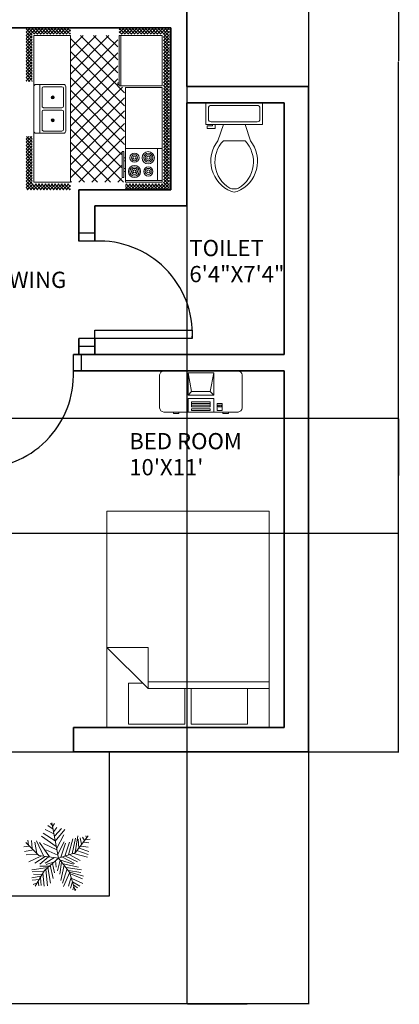
# Model space of a CAD drawing. Units: inches. Extents: x 4159 to 4826, y 299 to 1026.
# Tile 34 of 37: x 4685 to 4826, y 299 to 663. Entities that reach past the tile are written whole.
import ezdxf

# ---------------------------------------------------------------- set-up
doc = ezdxf.new("R2010")
doc.units = ezdxf.units.IN
for name, color, linetype, lineweight in [('A-ANNO-DIMS', 2, 'Continuous', 18), ('A-AREA-IDEN', 7, 'Continuous', 18), ('A-DOOR', 4, 'Continuous', 25), ('A-EQPM', 8, 'Continuous', 13), ('A-FLOR-BALC', 7, 'Continuous', 25), ('A-FLOR-FIXT', 9, 'Continuous', 18), ('A-FURN', 8, 'Continuous', 18), ('A-WALL', 7, 'Continuous', 35), ('L-PLNT', 94, 'Continuous', 13)]:
    doc.layers.add(name, color=color, linetype=linetype, lineweight=lineweight)
doc.styles.get("Standard").update_dxf_attribs({"font": 'arial.ttf'})
doc.dimstyles.get("Standard").update_dxf_attribs({"dimtxt": 0.18, "dimasz": 0.18, "dimexe": 0.18, "dimexo": 0.0625, "dimgap": 0.09, "dimtad": 0, "dimtih": 1, "dimtoh": 1, "dimdec": 4, "dimzin": 0, "dimdsep": 46, "dimtxsty": 'Standard', "dimcen": 0.09, "dimadec": 0, "dimazin": 0, "dimtfac": 1, "dimtdec": 4, "dimtofl": 0, "dimtmove": 0, "dimatfit": 3, "dimfxl": 1, "dimtolj": 1, "dimtzin": 0, "dimarcsym": 0})

# ---------------------------------------------------------------- blocks, each defined once
blk = doc.blocks.new('Bed - Queen')
for p, q in [((0, -80.00003), (0, 0)), ((0, 0), (59.99999, 0)), ((59.99999, 0), (59.99999, -80.00003)), ((7.99999, -1.2), (28.79998, -1.2)), ((7.99999, -14.4), (7.99999, -1.2)), ((28.79998, -1.2), (28.79998, -14.4)), ((31.19999, -1.2), (51.99999, -1.2)), ((31.19999, -14.4), (31.19999, -1.2)), ((51.99999, -1.2), (51.99999, -16.4)), ((0, -14.4), (44.8, -14.4)), ((59.99999, -29.6), (44.8, -14.4)), ((44.8, -14.4), (44.8, -29.6)), ((44.8, -16.8), (0, -16.8)), ((51.99999, -16.4), (46.79936, -16.4)), ((44.8, -29.6), (59.99999, -29.6)), ((59.99999, -80.00003), (0, -80.00003))]:
    blk.add_line(p, q)
blk = doc.blocks.new('Toilet - top')
for p, q in [((9.5, -6), (9.5, -2)), ((-10, -8.5), (-8, -8.5)), ((-10, -9.5), (-10, -8.5)), ((-7, -9.5), (-10, -9.5)), ((-8, -8.5), (-8, -8)), ((-7, -8), (-7, -9.5)), ((-4, -8), (-6, -14)), ((4, -8), (6, -14)), ((4, -14), (-4, -14))]:
    blk.add_line(p, q)
blk.add_lwpolyline([(10.5, -8), (10.5, 0), (-10.5, 0), (-10.5, -8)], close=True)
for points in [[(-9.5, -2), (-9.5, -6)], [(8.5, -1), (-8.5, -1)], [(-8.5, -7), (8.5, -7)]]:
    blk.add_lwpolyline(points)
for centre, radius, start, end in [((-8.62, -1.88), 0.884, 81.8699, 188.1301), ((8.62, -1.88), 0.884, 351.8699, 98.1301), ((-8.62, -6.12), 0.884, 171.8699, 278.1301), ((8.62, -6.12), 0.884, 261.8699, 8.1301), ((3.52, -21.58), 12.17, 141.4691, 247.9714), ((4.2, -21.82), 11.33, 136.3677, 238.9468), ((-3.52, -21.58), 12.17, 292.0284, 38.5307), ((-4.2, -21.82), 11.33, 301.053, 43.6321), ((0, -27.88), 4, 245.7318, 294.2682), ((0, -29), 4, 254.8605, 285.1395)]:
    blk.add_arc(centre, radius, start, end)
blk = doc.blocks.new('Desk - 30 x 60 in.')
for p, q in [((-26.999995, 0), (26.999995, 0)), ((-29.999995, -27), (-29.999995, -3)), ((29.999995, -3), (29.999995, -27)), ((26.999995, -30), (-26.999995, -30)), ((-20.000005, -30), (-20.000005, -31)), ((-20.000005, -31), (-16.000005, -31)), ((-16.000005, -31), (-16.000005, -30)), ((15.999995, -31), (15.999995, -30)), ((19.999995, -31), (15.999995, -31)), ((19.999995, -30), (19.999995, -31))]:
    blk.add_line(p, q)
for centre, start, end in [((-26.499995, -3.5), 98.1301, 171.8699), ((26.499995, -3.5), 8.130102, 81.8699), ((-26.499995, -26.5), 188.1301, 261.8699), ((26.499995, -26.5), 278.1301, 351.8699)]:
    blk.add_arc(centre, 3.535534, start, end)
blk = doc.blocks.new('Computer Terminal')
for p, q in [((-10, 11.5), (5, 11.5)), ((-8, 0.5), (-10, 11.5)), ((-10, -1.5), (-10, 11.5)), ((5, 11.5), (3, 0.5)), ((5, 11.5), (5, -1.5)), ((-10, -1.5), (-8, 0.5)), ((3, 0.5), (-8, 0.5)), ((3, 0.5), (5, -1.5)), ((5, -1.5), (-10, -1.5)), ((-10, -11.5), (-10, -3.5)), ((-10, -3.5), (5, -3.5)), ((-8, -5.5), (-8, -8.5)), ((3, -5.5), (-8, -5.5)), ((3, -8.5), (3, -5.5)), ((5, -3.5), (5, -11.5)), ((5, -11.5), (-10, -11.5)), ((3, -6.5), (-8, -6.5)), ((-8, -7.5), (3, -7.5)), ((-8, -8.5), (3, -8.5)), ((-8, -9.5), (-8, -10.5)), ((3, -9.5), (-8, -9.5)), ((-8, -10.5), (3, -10.5)), ((3, -10.5), (3, -9.5)), ((10, -6.5), (7, -6.5)), ((7, -6.5), (7, -10.5)), ((7, -10.5), (10, -10.5)), ((9.5, -7.5), (7.5, -7.5)), ((7.5, -7.5), (7.5, -8.5)), ((7.5, -8.5), (9.5, -8.5)), ((8.5, -7.5), (8.5, -8.5)), ((9.5, -8.5), (9.5, -7.5)), ((10, -10.5), (10, -6.5))]:
    blk.add_line(p, q)
blk = doc.blocks.new('Kitchen Layout - 7 x 8 ft')
for p, q in [((-5, 81.32), (2.68, 89)), ((-5, 83.44), (0.56, 89)), ((-5, 85.56), (-1.56, 89)), ((-5, 87.68), (-3.68, 89)), ((-1, 84.97), (-5, 88.97)), ((-1, 82.85), (-5, 86.85)), ((-1, 80.73), (-5, 84.73)), ((1.09, 85), (-2.91, 89)), ((3.21, 85), (-0.79, 89)), ((0.81, 85), (4.81, 89)), ((5.34, 85), (1.34, 89)), ((2.93, 85), (6.93, 89)), ((7.46, 85), (3.46, 89)), ((5.05, 85), (9.05, 89)), ((9.58, 85), (5.58, 89)), ((7.17, 85), (11.17, 89)), ((11.7, 85), (7.7, 89)), ((9.29, 85), (13.29, 89)), ((13.82, 85), (9.82, 89)), ((11.41, 85), (15.41, 89)), ((15.94, 85), (11.94, 89)), ((13.53, 85), (17.53, 89)), ((18.06, 85), (14.06, 89)), ((15.65, 85), (19.65, 89)), ((20.18, 85), (16.18, 89)), ((17.78, 85), (21.78, 89)), ((22.31, 85), (18.31, 89)), ((19.9, 85), (23.9, 89)), ((24.43, 85), (20.43, 89)), ((22.02, 85), (26.02, 89)), ((26.55, 85), (22.55, 89)), ((24.14, 85), (28.14, 89)), ((28.67, 85), (24.67, 89)), ((26.26, 85), (30.26, 89)), ((30.79, 85), (26.79, 89)), ((28.38, 85), (32.38, 89)), ((32.91, 85), (28.91, 89)), ((30.5, 85), (34.5, 89)), ((35.03, 85), (31.03, 89)), ((32.63, 85), (36.63, 89)), ((37.16, 85), (33.16, 89)), ((34, 84), (96, 84)), ((34, 60), (34, 84)), ((34.75, 85), (38.75, 89)), ((39.28, 85), (35.28, 89)), ((36.87, 85), (40.87, 89)), ((41.4, 85), (37.4, 89)), ((38.99, 85), (42.99, 89)), ((43.52, 85), (39.52, 89)), ((41.11, 85), (45.11, 89)), ((45.64, 85), (41.64, 89)), ((43.23, 85), (47.23, 89)), ((47.76, 85), (43.76, 89)), ((45.35, 85), (49.35, 89)), ((49.88, 85), (45.88, 89)), ((47.47, 85), (51.47, 89)), ((52, 85), (48, 89)), ((49.6, 85), (53.6, 89)), ((54.13, 85), (50.13, 89)), ((51.72, 85), (55.72, 89)), ((56.25, 85), (52.25, 89)), ((53.84, 85), (57.84, 89)), ((58.37, 85), (54.37, 89)), ((55.96, 85), (59.96, 89)), ((60.49, 85), (56.49, 89)), ((58.08, 85), (62.08, 89)), ((62.61, 85), (58.61, 89)), ((60.2, 85), (64.2, 89)), ((64.73, 85), (60.73, 89)), ((62.32, 85), (66.32, 89)), ((66.85, 85), (62.85, 89)), ((64.45, 85), (68.45, 89)), ((68.97, 85), (64.97, 89)), ((66.57, 85), (70.57, 89)), ((71.1, 85), (67.1, 89)), ((68.69, 85), (72.69, 89)), ((73.22, 85), (69.22, 89)), ((70.81, 85), (74.81, 89)), ((75.34, 85), (71.34, 89)), ((72.93, 85), (76.93, 89)), ((77.46, 85), (73.46, 89)), ((75.05, 85), (79.05, 89)), ((79.58, 85), (75.58, 89)), ((77.17, 85), (81.17, 89)), ((81.7, 85), (77.7, 89)), ((79.29, 85), (83.29, 89)), ((83.82, 85), (79.82, 89)), ((81.42, 85), (85.42, 89)), ((85.95, 85), (81.95, 89)), ((83.54, 85), (87.54, 89)), ((88.07, 85), (84.07, 89)), ((85.66, 85), (89.66, 89)), ((90.19, 85), (86.19, 89)), ((87.78, 85), (91.78, 89)), ((92.31, 85), (88.31, 89)), ((89.9, 85), (93.9, 89)), ((94.43, 85), (90.43, 89)), ((92.02, 85), (96.02, 89)), ((96.55, 85), (92.55, 89)), ((94.14, 85), (98.14, 89)), ((101, 82.67), (94.67, 89)), ((96, 84), (96, 60)), ((96.27, 85), (100.27, 89)), ((101, 84.79), (96.79, 89)), ((97, 83.61), (101, 87.61)), ((97, 81.49), (101, 85.49)), ((101, 80.55), (97, 84.55)), ((101, 86.92), (98.92, 89)), ((-5, 79.19), (-1, 83.19)), ((-1, 78.61), (-5, 82.61)), ((-5, 77.07), (-1, 81.07)), ((-1, 76.49), (-5, 80.49)), ((-5, 74.95), (-1, 78.95)), ((-1, 74.36), (-5, 78.36)), ((74, 81), (95, 81)), ((97, 79.37), (101, 83.37)), ((101, 78.43), (97, 82.43)), ((97, 77.25), (101, 81.25)), ((101, 76.31), (97, 80.31)), ((97, 75.13), (101, 79.13)), ((101, 74.19), (97, 78.19)), ((-5, 72.83), (-1, 76.83)), ((-1, 72.24), (-5, 76.24)), ((-5, 70.71), (-1, 74.71)), ((-1, 70.12), (-5, 74.12)), ((-5, 68.59), (-1, 72.59)), ((-1, 68), (-5, 72)), ((97, 73.01), (101, 77.01)), ((101, 72.07), (97, 76.07)), ((97, 70.89), (101, 74.89)), ((101, 69.95), (97, 73.95)), ((97, 68.76), (101, 72.76)), ((101, 67.82), (97, 71.82)), ((-5, 66.47), (-1, 70.47)), ((-1, 65.88), (-5, 69.88)), ((-5, 64.35), (-1, 68.35)), ((-1, 63.76), (-5, 67.76)), ((-5, 62.22), (-1, 66.22)), ((-1, 61.64), (-5, 65.64)), ((97, 66.64), (101, 70.64)), ((101, 65.7), (97, 69.7)), ((97, 64.52), (101, 68.52)), ((101, 63.58), (97, 67.58)), ((97, 62.4), (101, 66.4)), ((101, 61.46), (97, 65.46)), ((-5, 60.1), (-1, 64.1)), ((-1, 59.52), (-5, 63.52)), ((-5, 57.98), (-1, 61.98)), ((-1, 57.39), (-5, 61.39)), ((-1.73, 56), (-5, 59.27)), ((-4.86, 56), (-1, 59.86)), ((10.4, 24), (45.9, 59.5)), ((18.88, 24), (54.38, 59.5)), ((27.37, 24), (62.87, 59.5)), ((33.03, 55.11), (37.41, 59.5)), ((96, 60), (34, 60)), ((35.85, 24), (71.35, 59.5)), ((76.2, 24), (40.7, 59.5)), ((84.68, 24), (49.18, 59.5)), ((93.17, 24), (57.67, 59.5)), ((61.31, 24), (96, 58.69)), ((96, 29.65), (66.15, 59.5)), ((80, 60), (80, 59)), ((82, 59), (82, 60)), ((87, 59), (87, 60)), ((89, 60), (89, 59)), ((97, 60.28), (101, 64.28)), ((100.34, 60), (97, 63.34)), ((98.22, 60), (97, 61.22)), ((98.84, 60), (101, 62.16)), ((100.96, 60), (101, 60.04)), ((-3.85, 56), (-5, 57.15)), ((-2.74, 56), (-1, 57.74)), ((0, 57), (33, 57)), ((0, 30.57), (24.43, 55)), ((0, 39.06), (15.94, 55)), ((0, 47.54), (7.46, 55)), ((1.91, 24), (32.91, 55)), ((33.77, 24), (2.77, 55)), ((42.26, 24), (11.26, 55)), ((50.74, 24), (19.74, 55)), ((59.23, 24), (28.23, 55)), ((31, 55), (31, 56)), ((32, 55), (31, 55)), ((32, 56), (32, 55)), ((67.71, 24), (33.68, 58.04)), ((44.34, 24), (77.84, 57.5)), ((52.82, 24), (86.32, 57.5)), ((96, 38.14), (76.64, 57.5)), ((96, 46.63), (85.13, 57.5)), ((96, 55.11), (93.57, 57.54)), ((25.29, 24), (0, 49.29)), ((69.79, 24), (96, 50.21)), ((16.8, 24), (0, 40.8)), ((78.28, 24), (96, 41.72)), ((8.32, 24), (0, 32.32)), ((86.76, 24), (96, 33.24)), ((-5, 21.92), (-2.92, 24)), ((-5, 19.8), (-1, 23.8)), ((-1, 19.21), (-5, 23.21)), ((-5, 17.68), (-1, 21.68)), ((-1, 17.09), (-5, 21.09)), ((-5, 15.55), (-1, 19.55)), ((-1, 21.33), (-3.67, 24)), ((-1, 23.45), (-1.55, 24)), ((0, 24), (96, 24)), ((0, 0), (0, 24)), ((95.25, 24), (96, 24.75)), ((96, 24), (96, 0)), ((97, 22.1), (98.9, 24)), ((97, 19.97), (101, 23.97)), ((101, 19.03), (97, 23.03)), ((97, 17.85), (101, 21.85)), ((101, 16.91), (97, 20.91)), ((97, 15.73), (101, 19.73)), ((101, 21.16), (98.16, 24)), ((101, 23.28), (100.28, 24)), ((-1, 14.97), (-5, 18.97)), ((-5, 13.43), (-1, 17.43)), ((-1, 12.85), (-5, 16.85)), ((-5, 11.31), (-1, 15.31)), ((-1, 10.73), (-5, 14.73)), ((-5, 9.19), (-1, 13.19)), ((47.25, 6.5), (47.25, 18.5)), ((48.75, 18.5), (48.75, 6.5)), ((101, 14.79), (97, 18.79)), ((97, 13.61), (101, 17.61)), ((101, 12.67), (97, 16.67)), ((97, 11.49), (101, 15.49)), ((101, 10.55), (97, 14.55)), ((97, 9.37), (101, 13.37)), ((-1, 8.6), (-5, 12.6)), ((-5, 7.07), (-1, 11.07)), ((-1, 6.48), (-5, 10.48)), ((-5, 4.95), (-1, 8.95)), ((-1, 4.36), (-5, 8.36)), ((-5, 2.83), (-1, 6.83)), ((101, 8.43), (97, 12.43)), ((97, 7.25), (101, 11.25)), ((101, 6.31), (97, 10.31)), ((97, 5.12), (101, 9.12)), ((101, 4.18), (97, 8.18)), ((97, 3), (101, 7)), ((-1, 2.24), (-5, 6.24)), ((-5, 0.71), (-1, 4.71)), ((-1, 0.12), (-5, 4.12)), ((-5, -1.42), (-1, 2.58)), ((2, -5), (-5, 2)), ((-5, -3.54), (-1, 0.46)), ((96, 0), (0, 0)), ((64, 4), (32, 4)), ((93.24, -5), (101, 2.76)), ((95.36, -5), (101, 0.64)), ((101, 2.06), (97, 6.06)), ((97, 0.88), (101, 4.88)), ((101, -0.06), (97, 3.94)), ((101, -2.18), (97, 1.82)), ((-0.12, -5), (-5, -0.12)), ((-2.25, -5), (-5, -2.25)), ((-4.37, -5), (-5, -4.37)), ((-4.34, -5), (-0.34, -1)), ((-2.22, -5), (1.78, -1)), ((-0.1, -5), (3.9, -1)), ((4.12, -5), (0.12, -1)), ((2.02, -5), (6.02, -1)), ((6.24, -5), (2.24, -1)), ((4.14, -5), (8.14, -1)), ((8.36, -5), (4.36, -1)), ((6.27, -5), (10.27, -1)), ((10.48, -5), (6.48, -1)), ((8.39, -5), (12.39, -1)), ((12.6, -5), (8.6, -1)), ((10.51, -5), (14.51, -1)), ((14.73, -5), (10.73, -1)), ((12.63, -5), (16.63, -1)), ((16.85, -5), (12.85, -1)), ((14.75, -5), (18.75, -1)), ((18.97, -5), (14.97, -1)), ((16.87, -5), (20.87, -1)), ((21.09, -5), (17.09, -1)), ((18.99, -5), (22.99, -1)), ((23.21, -5), (19.21, -1)), ((21.11, -5), (25.11, -1)), ((25.33, -5), (21.33, -1)), ((23.24, -5), (27.24, -1)), ((27.45, -5), (23.45, -1)), ((25.36, -5), (29.36, -1)), ((29.57, -5), (25.57, -1)), ((27.48, -5), (30, -2.48)), ((30, -3.3), (27.7, -1)), ((29.6, -5), (30, -4.6)), ((30, -1.18), (29.82, -1)), ((66, -2.54), (67.54, -1)), ((66, -4.66), (69.66, -1)), ((69.88, -5), (66, -1.12)), ((67.76, -5), (66, -3.24)), ((67.78, -5), (71.78, -1)), ((72, -5), (68, -1)), ((69.9, -5), (73.9, -1)), ((74.12, -5), (70.12, -1)), ((72.03, -5), (76.03, -1)), ((76.24, -5), (72.24, -1)), ((74.15, -5), (78.15, -1)), ((78.36, -5), (74.36, -1)), ((76.27, -5), (80.27, -1)), ((80.49, -5), (76.49, -1)), ((78.39, -5), (82.39, -1)), ((82.61, -5), (78.61, -1)), ((80.51, -5), (84.51, -1)), ((84.73, -5), (80.73, -1)), ((82.63, -5), (86.63, -1)), ((86.85, -5), (82.85, -1)), ((84.75, -5), (88.75, -1)), ((88.97, -5), (84.97, -1)), ((86.88, -5), (90.88, -1)), ((91.09, -5), (87.09, -1)), ((89, -5), (93, -1)), ((93.21, -5), (89.21, -1)), ((91.12, -5), (95.12, -1)), ((95.34, -5), (91.34, -1)), ((97.46, -5), (93.46, -1)), ((99.58, -5), (95.58, -1)), ((101, -4.3), (97, -0.3)), ((97.48, -5), (101, -1.48)), ((99.6, -5), (101, -3.6))]:
    blk.add_line(p, q)
for points in [[(0, 56), (0, 84), (33, 84), (33, 56)], [(74, 60), (74, 84), (95, 84), (95, 60)], [(76, 58), (76, 59), (93, 59), (93, 58)]]:
    blk.add_lwpolyline(points, close=True)
for points in [[(32, 1.5), (32, 19.5)], [(33.5, 21), (62.5, 21)], [(34.5, 19.5), (46.25, 19.5)], [(49.75, 19.5), (61.5, 19.5)], [(64, 19.5), (64, 1.5)], [(33.5, 6.5), (33.5, 18.5)], [(62.5, 18.5), (62.5, 6.5)], [(62.5, 0), (33.5, 0)], [(46.25, 5.5), (34.5, 5.5)], [(61.5, 5.5), (49.75, 5.5)]]:
    blk.add_lwpolyline(points)
for centre, radius in [((80, 75), 4), ((80, 75), 3), ((89, 75), 3), ((80, 75), 2), ((80, 75), 1), ((89, 75), 2), ((89, 75), 1), ((80, 66), 3), ((80, 66), 2), ((80, 66), 1), ((89, 66), 4), ((89, 66), 3), ((89, 66), 2), ((89, 66), 1), ((40.5, 12.5), 1), ((40.5, 12.5), 0.5), ((55.5, 12.5), 1), ((55.5, 12.5), 0.5)]:
    blk.add_circle(centre, radius)
for centre, radius, start, end in [((33.5, 19.5), 1.5, 90, 180), ((34.5, 18.5), 1, 90, 180), ((46.25, 18.5), 1, 0, 90), ((49.75, 18.5), 1, 90, 180), ((61.5, 18.5), 1, 0, 90), ((62.5, 19.5), 1.5, 0, 90), ((34.5, 6.5), 1, 180, 270), ((46.25, 6.5), 1, 270, 0), ((49.75, 6.5), 1, 180, 270), ((61.5, 6.5), 1, 270, 0), ((33.5, 1.5), 1.5, 180, 270), ((62.5, 1.5), 1.5, 270, 0)]:
    blk.add_arc(centre, radius, start, end)
blk = doc.blocks.new('*U12')
for p, q in [((-8.737, 47.138), (-17.069, 52.711)), ((-10.186, 53.64), (-13.084, 55.962)), ((0, 0), (-10.5, 57)), ((-9.099, 51.782), (-6.563, 55.962)), ((-7.65, 43.423), (-2.578, 49.46)), ((-5.839, 35.992), (4.667, 48.067)), ((-3.665, 19.273), (-27.574, 35.527)), ((-5.114, 28.097), (-24.676, 40.636)), ((-7.288, 39.707), (-21.778, 46.673)), ((-5.114, 27.632), (10.463, 46.673)), ((-2.941, 16.486), (8.652, 37.85)), ((22.055, 7.198), (27.489, 32.277)), ((27, 9), (48, 36)), ((27.127, 9.056), (31.112, 35.992)), ((35.096, 32.741), (37.27, 22.524)), ((38.719, 34.134), (41.979, 28.561)), ((44.153, 36.456), (45.239, 32.741)), ((-47.498, 19.737), (-55.83, 18.344)), ((-31.5, 4.5), (-52.5, 25.5)), ((-48.585, 21.131), (-49.309, 29.026)), ((-43.513, 28.561), (-42.427, 15.558)), ((-38.442, 26.239), (-34.819, 7.663)), ((-35.544, 28.097), (-24.314, 3.947)), ((-14.533, 2.09), (-30.834, 25.31)), ((-24.314, 23.917), (-2.941, 13.7)), ((-1.129, 6.734), (9.014, 26.704)), ((3.942, 1.625), (11.187, 24.381)), ((10.101, 3.483), (17.708, 26.239)), ((16.259, 5.805), (23.142, 31.348)), ((31.836, 30.883), (32.561, 16.486)), ((33.285, 16.486), (48.862, 10.913)), ((36.183, 19.737), (48.137, 17.88)), ((40.53, 25.775), (48.862, 24.846)), ((43.791, 29.954), (51.036, 30.883)), ((-40.615, 13.7), (-55.105, 10.913)), ((-33.37, 6.269), (-52.207, 5.34)), ((-28.299, 3.483), (-47.86, -5.805)), ((-21.416, 3.018), (-38.079, -8.128)), ((0, 0), (-31.5, 4.5)), ((-15.982, 2.09), (-30.11, -9.521)), ((0, 0), (-22.5, -19.5)), ((-6.563, 1.161), (-21.416, -8.128)), ((-20.691, 13.7), (-1.129, 4.876)), ((0, 0), (27, 9)), ((0, 0), (18, -22.5)), ((6.478, 1.625), (26.04, -8.592)), ((11.187, 3.483), (30.749, -5.805)), ((18.07, 5.805), (35.096, -3.483)), ((24.229, 7.663), (46.688, 1.625)), ((29.662, 12.307), (48.137, 6.269)), ((-17.431, -15.094), (-42.789, -18.809)), ((-15.257, -12.772), (-30.11, -12.772)), ((-6.563, -5.805), (-19.967, -9.985)), ((-17.069, -15.094), (-12.721, -40.172)), ((-13.446, -11.378), (-8.737, -32.741)), ((-9.461, -8.592), (-6.201, -23.453)), ((-4.752, -3.483), (-3.665, -14.629)), ((2.493, -3.019), (-1.491, -20.202)), ((1.769, -2.555), (24.229, -9.521)), ((5.029, -6.27), (2.131, -25.775)), ((9.014, -11.378), (3.58, -35.992)), ((7.565, -9.056), (32.198, -14.629)), ((12.274, -15.094), (36.907, -18.809)), ((-28.299, -29.026), (-42.789, -31.348)), ((-24.314, -21.596), (-42.427, -22.06)), ((-26.849, -26.24), (-40.253, -25.775)), ((-22.5, -19.5), (-37.5, -45)), ((-29.023, -30.884), (-27.936, -43.887)), ((-25.038, -23.918), (-22.865, -45.281)), ((-20.691, -18.345), (-17.793, -44.352)), ((14.085, -16.951), (6.478, -40.172)), ((18.07, -22.524), (8.289, -45.745)), ((20.244, -30.419), (15.897, -44.816)), ((16.259, -19.738), (36.183, -22.989)), ((18, -22.5), (27, -52.5)), ((18.433, -22.524), (40.53, -29.026)), ((19.157, -25.311), (38.719, -33.206)), ((-30.834, -34.135), (-42.427, -35.528)), ((-34.457, -39.708), (-40.978, -42.494)), ((-32.646, -36.921), (-31.921, -44.352)), ((22.78, -37.85), (19.519, -48.532)), ((21.331, -32.741), (39.081, -40.636)), ((22.78, -38.314), (34.372, -44.816)), ((24.591, -45.745), (23.142, -50.854)), ((24.591, -43.423), (30.749, -47.603)), ((26.764, -49.925), (28.213, -50.854))]:
    blk.add_line(p, q)
blk = doc.blocks.new('DOOR-SWING-36IN')
blk.add_lwpolyline([(0, 0), (-3, 0), (-3, 36), (0, 36)], close=True)
blk.add_arc((-1.5, 1.5), 34.53, 87.5104, 182.4896)
blk = doc.blocks.new('DOOR-FRAME-36IN')
for p, q in [((0, 6), (0, 0)), ((3, 6), (3, 0)), ((39, 6), (39, 0)), ((42, 6), (42, 0))]:
    blk.add_line(p, q)
blk = doc.blocks.new('*D45')
at = {"layer": 'A-ANNO-DIMS', "color": 0, "lineweight": -2, "transparency": 16777216}
for p, q in [((4792.37, 903.25), (4825.74, 903.25)), ((4825.56, 903.07), (4825.56, 647.94)), ((4825.56, 392.43), (4825.56, 647.57)), ((4792.37, 392.25), (4825.74, 392.25))]:
    blk.add_line(p, q, dxfattribs=at)
at = {"layer": 'A-ANNO-DIMS', "color": 0, "transparency": 16777216}
for points in [[(4825.53, 903.07), (4825.59, 903.07), (4825.56, 903.25)], [(4825.53, 392.43), (4825.59, 392.43), (4825.56, 392.25)]]:
    blk.add_solid(points, dxfattribs=at)
at = {"layer": 'Defpoints', "color": 0, "transparency": 16777216}
for p in [(4792.31, 903.25), (4792.31, 392.25), (4825.56, 392.25)]:
    blk.add_point(p, dxfattribs=at)
at = {"layer": 'A-ANNO-DIMS', "color": 0, "transparency": 16777216, "insert": (4825.56, 647.75), "char_height": 0.18, "attachment_point": 5}
blk.add_mtext('\\A1;511', dxfattribs=at)
blk = doc.blocks.new('*D48')
at = {"layer": 'A-ANNO-DIMS', "color": 0, "lineweight": -2, "transparency": 16777216}
for p, q in [((4792.31, 392.19), (4792.31, 298.77)), ((4547.89, 332.13), (4547.89, 298.77)), ((4548.07, 298.95), (4669.7, 298.95)), ((4792.13, 298.95), (4670.49, 298.95))]:
    blk.add_line(p, q, dxfattribs=at)
at = {"layer": 'A-ANNO-DIMS', "color": 0, "transparency": 16777216}
for points in [[(4548.07, 298.98), (4548.07, 298.92), (4547.89, 298.95)], [(4792.13, 298.98), (4792.13, 298.92), (4792.31, 298.95)]]:
    blk.add_solid(points, dxfattribs=at)
at = {"layer": 'Defpoints', "color": 0, "transparency": 16777216}
for p in [(4792.31, 392.25), (4547.89, 332.2), (4792.31, 298.95)]:
    blk.add_point(p, dxfattribs=at)
at = {"layer": 'A-ANNO-DIMS', "color": 0, "transparency": 16777216, "insert": (4670.1, 298.95), "char_height": 0.18, "attachment_point": 5}
blk.add_mtext('\\A1;244.4', dxfattribs=at)
blk = doc.blocks.new('*D49')
at = {"layer": 'A-ANNO-DIMS', "color": 0, "lineweight": -2, "transparency": 16777216}
for p, q in [((4747.31, 693.73), (4747.31, 298.77)), ((4792.31, 693.73), (4792.31, 298.77)), ((4747.49, 298.95), (4769.59, 298.95)), ((4792.13, 298.95), (4770.03, 298.95))]:
    blk.add_line(p, q, dxfattribs=at)
at = {"layer": 'A-ANNO-DIMS', "color": 0, "transparency": 16777216}
for points in [[(4747.49, 298.98), (4747.49, 298.92), (4747.31, 298.95)], [(4792.13, 298.98), (4792.13, 298.92), (4792.31, 298.95)]]:
    blk.add_solid(points, dxfattribs=at)
at = {"layer": 'Defpoints', "color": 0, "transparency": 16777216}
for p in [(4747.31, 693.79), (4792.31, 693.79), (4792.31, 298.95)]:
    blk.add_point(p, dxfattribs=at)
at = {"layer": 'A-ANNO-DIMS', "color": 0, "transparency": 16777216, "insert": (4769.81, 298.95), "char_height": 0.18, "attachment_point": 5}
blk.add_mtext('\\A1;45', dxfattribs=at)
blk = doc.blocks.new('*D54')
at = {"layer": 'A-ANNO-DIMS', "color": 0, "lineweight": -2, "transparency": 16777216}
for p, q in [((4501.37, 515.71), (4825.74, 515.71)), ((4825.56, 515.53), (4825.56, 494.64)), ((4825.56, 473.38), (4825.56, 494.27)), ((4541.95, 473.2), (4825.74, 473.2))]:
    blk.add_line(p, q, dxfattribs=at)
at = {"layer": 'A-ANNO-DIMS', "color": 0, "transparency": 16777216}
for points in [[(4825.53, 515.53), (4825.59, 515.53), (4825.56, 515.71)], [(4825.53, 473.38), (4825.59, 473.38), (4825.56, 473.2)]]:
    blk.add_solid(points, dxfattribs=at)
at = {"layer": 'Defpoints', "color": 0, "transparency": 16777216}
for p in [(4501.31, 515.71), (4825.56, 515.71), (4541.89, 473.2)]:
    blk.add_point(p, dxfattribs=at)
at = {"layer": 'A-ANNO-DIMS', "color": 0, "transparency": 16777216, "insert": (4825.56, 494.45), "char_height": 0.18, "attachment_point": 5}
blk.add_mtext('\\A1;42.52', dxfattribs=at)

msp = doc.modelspace()

# ---------------------------------------------------------------- linework, layer by layer
at = {"layer": 'A-FLOR-BALC'}
msp.add_lwpolyline([(4591.233, 392.254), (4718.606, 392.254), (4718.606, 338.75), (4591.233, 338.75)], close=True, dxfattribs=at)
at = {"layer": 'A-WALL'}
for p, q in [((4747.31, 638.43), (4747.31, 693.788)), ((4741.31, 660.254), (4547.889, 660.254)), ((4741.31, 600.254), (4741.31, 660.254)), ((4747.31, 638.43), (4792.31, 638.43)), ((4747.31, 594.254), (4747.31, 632.43)), ((4747.31, 632.43), (4783.31, 632.43)), ((4783.31, 539.254), (4783.31, 632.43)), ((4741.31, 600.254), (4707.31, 600.254)), ((4707.31, 581.254), (4707.31, 600.254)), ((4747.31, 594.254), (4713.31, 594.254)), ((4713.31, 581.254), (4713.31, 594.254)), ((4707.31, 539.254), (4707.31, 545.254)), ((4713.31, 539.254), (4713.31, 545.254)), ((4783.31, 539.254), (4705.31, 539.254)), ((4783.31, 533.254), (4705.31, 533.254)), ((4783.31, 533.254), (4705.31, 533.254)), ((4783.31, 401.254), (4783.31, 533.254)), ((4783.31, 401.254), (4705.31, 401.254)), ((4783.31, 401.254), (4705.31, 401.254)), ((4705.31, 401.254), (4705.31, 392.254)), ((4792.31, 392.254), (4705.31, 392.254))]:
    msp.add_line(p, q, dxfattribs=at)
msp.add_lwpolyline([(4792.31, 392.254), (4792.31, 638.43)], dxfattribs=at)

# ---------------------------------------------------------------- block references
at = {"layer": 'A-DOOR'}
for name, p, rotation in [('DOOR-FRAME-36IN', (4707.31, 584.254), 270.0000000000003), ('DOOR-SWING-36IN', (4713.31, 545.254), 270.0000000000011), ('DOOR-FRAME-36IN', (4708.31, 539.254), 180), ('DOOR-SWING-36IN', (4669.31, 533.254), 180)]:
    msp.add_blockref(name, p, dxfattribs=dict(at, rotation=rotation))
at = {"layer": 'A-EQPM', "xscale": 0.6328414688201627, "yscale": 0.6328414688201627, "zscale": 0.6328414688201627}
msp.add_blockref('Computer Terminal', (4754.072, 525.235), dxfattribs=at)
at = {"layer": 'A-FLOR-FIXT', "xscale": 0.5650329326971529, "yscale": 0.5650329326971529, "zscale": 0.5650329326971529, "rotation": 270}
msp.add_blockref('Kitchen Layout - 7 x 8 ft', (4690.635, 657.322), dxfattribs=at)
at = {"layer": 'A-FLOR-FIXT'}
msp.add_blockref('Toilet - top', (4764.803, 632.43), dxfattribs=at)
at = {"layer": 'A-FURN', "xscale": 0.5098837128326598, "yscale": 0.5098837128326598, "zscale": 0.5098837128326598}
msp.add_blockref('Desk - 30 x 60 in.', (4752.49, 533.254), dxfattribs=at)
at = {"layer": 'A-FURN', "rotation": 180}
msp.add_blockref('Bed - Queen', (4777.729, 401.269), dxfattribs=at)
at = {"layer": 'L-PLNT', "xscale": 0.2292012274639507, "yscale": 0.2292012274639507, "zscale": 0.2292012274639507}
msp.add_blockref('*U12', (4699.815, 352.819), dxfattribs=at)

# ---------------------------------------------------------------- texts
at = {"layer": 'A-AREA-IDEN'}
for s, p in [('TOILET', (4748.223, 575.696)), ('6\'4"X7\'4"', (4748.223, 566.057)), ('DINING\\DRAWING', (4634.632, 563.924)), ('BED ROOM', (4725.992, 504.211)), ("10'X11'", (4725.992, 494.572))]:
    msp.add_text(s, height=6, dxfattribs=at).set_placement(p)

# ---------------------------------------------------------------- dimensions: what is measured, and where the dimension line sits
at = {"layer": 'A-ANNO-DIMS'}
for base, p1, p2, override, picture, middle in [((4825.56, 392.254), (4792.31, 903.254), (4792.31, 392.254), {"dimdec": 0, "dimlfac": 1, "dimrnd": 0, "dimzin": 0, "dimdsep": 46, "dimlunit": 2}, '*D45', (4825.56, 647.754)), ((4825.56, 515.713), (4541.889, 473.195), (4501.31, 515.713), {"dimdec": 2, "dimlfac": 1, "dimrnd": 0, "dimzin": 0, "dimdsep": 46, "dimlunit": 2}, '*D54', (4825.56, 494.454))]:
    dim = msp.add_linear_dim(base=base, p1=p1, p2=p2, angle=90, dimstyle='Standard', override=override, dxfattribs=at)
    dim.commit()
    dim.dimension.update_dxf_attribs({"geometry": picture, "text_midpoint": middle})
for p1, p2, override, picture, middle in [((4747.31, 693.788), (4792.31, 693.788), {"dimdec": 0, "dimlfac": 1, "dimrnd": 0, "dimzin": 0, "dimdsep": 46, "dimlunit": 2}, '*D49', (4769.81, 298.945)), ((4547.889, 332.195), (4792.31, 392.254), {"dimdec": 1, "dimlfac": 1, "dimrnd": 0, "dimzin": 0, "dimdsep": 46, "dimlunit": 2}, '*D48', (4670.1, 298.945))]:
    dim = msp.add_linear_dim(base=(4792.31, 298.945), p1=p1, p2=p2, dimstyle='Standard', override=override, dxfattribs=at)
    dim.commit()
    dim.dimension.update_dxf_attribs({"geometry": picture, "text_midpoint": middle})

doc.saveas('drawing.dxf')
